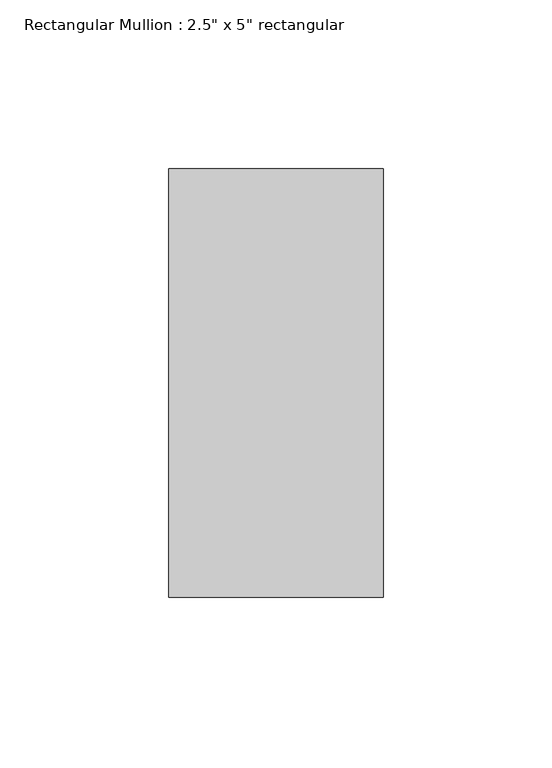
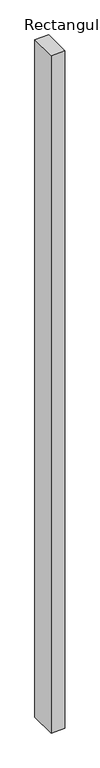
"""IFC4 building model written with IfcOpenShell, lengths in millimetres: member geometry."""

from ifc_helpers import new_model, si_unit, frame, origin, place, context, project, spatial, polyline, outline, extrude, source, transform, mapped, element, save


def member_dede372a(model_context):
    return source(origin(), model_context, "Body", "SweptSolid", [
        extrude(outline(polyline([(0.0, 63.5), (0.0, -63.5), (-63.5, -63.5), (-63.5, 63.5), (0.0, 63.5)])), frame((0.0, 0.0, -3263.9), z_axis=(0.0, 0.0, 1.0), x_axis=(1.0, 0.0, 0.0)), (0.0, 0.0, 1.0), 3263.9),
    ])


if __name__ == "__main__":
    model = new_model("IFC4")
    model_context = context("Model", 3, world=origin())
    ifc_project = project(units=[si_unit("LENGTHUNIT", "METRE", prefix="MILLI")], contexts=[model_context])
    site = spatial("IfcSite", under=ifc_project)
    building = spatial("IfcBuilding", under=site)
    placement = place(None, origin())
    member_shape = member_dede372a(model_context)
    element("IfcMember", 1, ObjectType="Rectangular Mullion : 2.5\" x 5\" rectangular", at=placement, inside=building, context=model_context, shape_type="MappedRepresentation", body=[
        mapped(member_shape, transform((0.0, 0.0, 0.0), x_axis=(1.0, 0.0, 0.0), y_axis=(0.0, 1.0, 0.0), z_axis=(0.0, 0.0, 1.0))),
    ])
    save(model, "model.ifc")

# Revit data of these elements
# Type "Rectangular Mullion : 2.5\" x 5\" rectangular"
#   built-in parameter 1007304 = 0.416667 (stored number, unit not read)
#   built-in parameter 1007301 = 0.104167 (stored number, unit not read)
#   built-in parameter 1007300 = 0.104167 (stored number, unit not read)
# Element 1 (IfcMember, "Rectangular Mullion : 2.5\" x 5\" rectangular")
#   Materials on its faces: "Iron, Ductile"
# Materials
#   "Iron, Ductile": class "Metal", colour RGB 0 0 0, transparency 0, Description = "Ductile cast iron", Cost = 0
